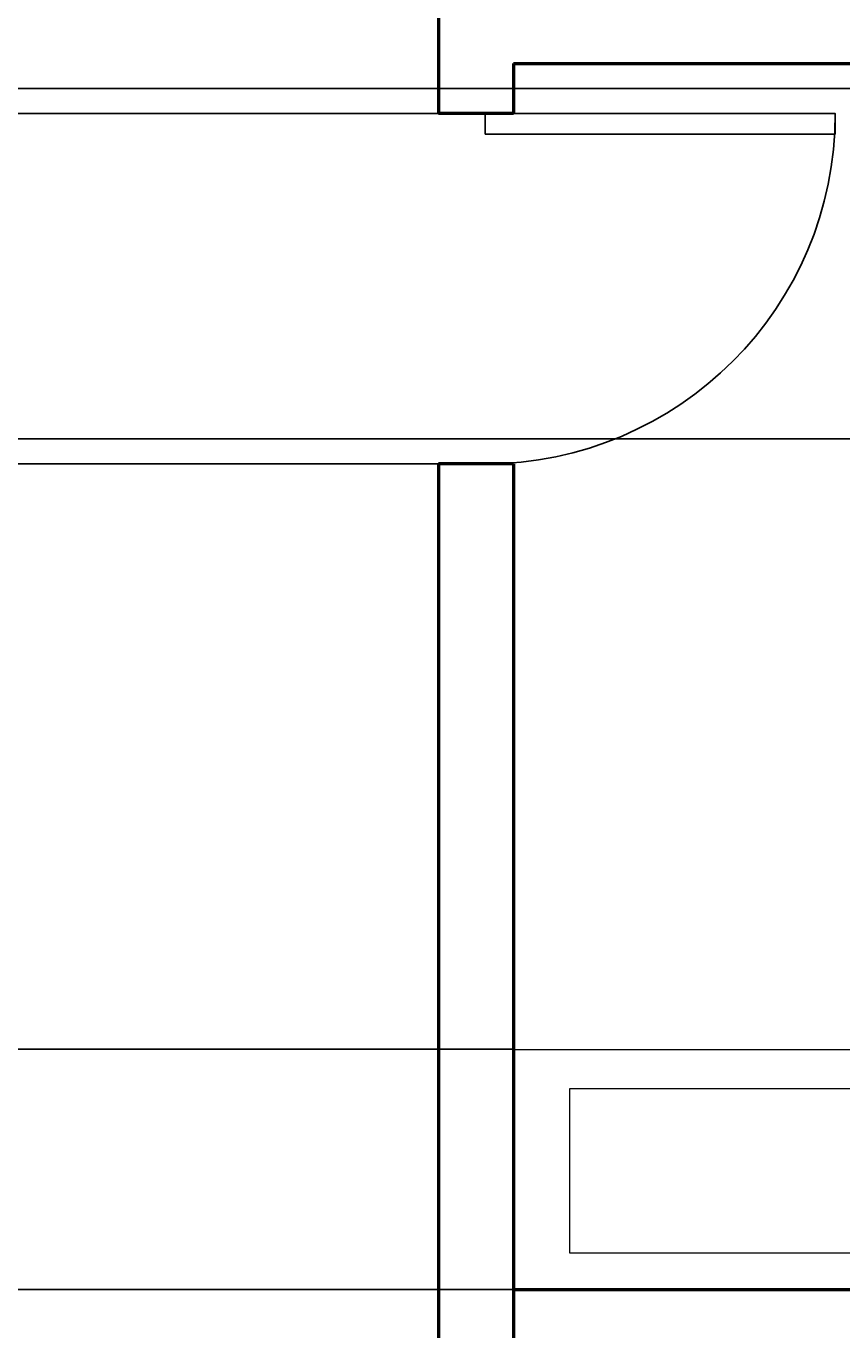
# Model space of a CAD drawing. Units: inches. Extents: x 5375 to 6084, y 16106 to 17259.
# Tile 27 of 32: x 5768 to 5866, y 16776 to 16932. Entities that reach past the tile are written whole.
import ezdxf

# ---------------------------------------------------------------- set-up
doc = ezdxf.new("R2010")
doc.units = ezdxf.units.IN
for name, color, linetype, lineweight in [('A-ANNO-DIMS', 2, 'Continuous', 18), ('A-FLOR-CASE', 3, 'Continuous', 18), ('A-FLOR-FIXT', 3, 'Continuous', 18), ('DOOR', 4, 'Continuous', 25), ('WALL', 6, 'Continuous', 50)]:
    doc.layers.add(name, color=color, linetype=linetype, lineweight=lineweight)
doc.styles.get("Standard").update_dxf_attribs({"font": 'arial.ttf'})
doc.dimstyles.get("Standard").update_dxf_attribs({"dimtxt": 0.18, "dimasz": 0.18, "dimexe": 0.18, "dimexo": 0.0625, "dimgap": 0.09, "dimtad": 0, "dimtih": 1, "dimtoh": 1, "dimdec": 4, "dimzin": 0, "dimdsep": 46, "dimtxsty": 'Standard', "dimcen": 0.09, "dimadec": 0, "dimazin": 0, "dimtfac": 1, "dimtdec": 4, "dimtofl": 0, "dimtmove": 0, "dimatfit": 3, "dimfxl": 1, "dimtolj": 1, "dimtzin": 0, "dimarcsym": 0})

# ---------------------------------------------------------------- blocks, each defined once
blk = doc.blocks.new('*U2')
for p, q in [((0, 0), (0, -100)), ((750, 0), (750, -100))]:
    blk.add_line(p, q)
blk.add_lwpolyline([(0, 0), (0, 750), (43.75, 750), (43.75, 0)], close=True)
blk.add_arc((0, 0), 750, 0, 90)
blk = doc.blocks.new('*D41')
at = {"layer": 'A-ANNO-DIMS', "color": 0, "lineweight": -2, "transparency": 16777216}
for p, q in [((5702.18, 16924.58), (6084.2, 16924.58)), ((6084.02, 16924.4), (6084.02, 16903.76)), ((6084.02, 16882.76), (6084.02, 16903.4)), ((5702.18, 16882.58), (6084.2, 16882.58))]:
    blk.add_line(p, q, dxfattribs=at)
at = {"layer": 'A-ANNO-DIMS', "color": 0, "transparency": 16777216}
for points in [[(6083.99, 16924.4), (6084.05, 16924.4), (6084.02, 16924.58)], [(6083.99, 16882.76), (6084.05, 16882.76), (6084.02, 16882.58)]]:
    blk.add_solid(points, dxfattribs=at)
at = {"layer": 'Defpoints', "color": 0, "transparency": 16777216}
for p in [(5702.12, 16924.58), (6084.02, 16924.58), (5702.12, 16882.58)]:
    blk.add_point(p, dxfattribs=at)
at = {"layer": 'A-ANNO-DIMS', "color": 0, "transparency": 16777216, "insert": (6084.02, 16903.58), "char_height": 0.18, "attachment_point": 5}
blk.add_mtext('\\A1;42', dxfattribs=at)
blk = doc.blocks.new('*D42')
at = {"layer": 'A-ANNO-DIMS', "color": 0, "lineweight": -2, "transparency": 16777216}
for p, q in [((5826.06, 16921.58), (5375.56, 16921.58)), ((5375.74, 16921.4), (5375.74, 16900.76)), ((5375.74, 16879.76), (5375.74, 16900.4)), ((5826.06, 16879.58), (5375.56, 16879.58))]:
    blk.add_line(p, q, dxfattribs=at)
at = {"layer": 'A-ANNO-DIMS', "color": 0, "transparency": 16777216}
for points in [[(5375.71, 16921.4), (5375.77, 16921.4), (5375.74, 16921.58)], [(5375.71, 16879.76), (5375.77, 16879.76), (5375.74, 16879.58)]]:
    blk.add_solid(points, dxfattribs=at)
at = {"layer": 'Defpoints', "color": 0, "transparency": 16777216}
for p in [(5826.12, 16921.58), (5375.74, 16879.58), (5826.12, 16879.58)]:
    blk.add_point(p, dxfattribs=at)
at = {"layer": 'A-ANNO-DIMS', "color": 0, "transparency": 16777216, "insert": (5375.74, 16900.58), "char_height": 0.18, "attachment_point": 5}
blk.add_mtext('\\A1;42', dxfattribs=at)
blk = doc.blocks.new('*D43')
at = {"layer": 'A-ANNO-DIMS', "color": 0, "lineweight": -2, "transparency": 16777216}
for p, q in [((5826.06, 16809.37), (5375.56, 16809.37)), ((5375.74, 16809.19), (5375.74, 16795.15)), ((5375.74, 16780.76), (5375.74, 16794.79)), ((5826.06, 16780.58), (5375.56, 16780.58))]:
    blk.add_line(p, q, dxfattribs=at)
at = {"layer": 'A-ANNO-DIMS', "color": 0, "transparency": 16777216}
for points in [[(5375.71, 16809.19), (5375.77, 16809.19), (5375.74, 16809.37)], [(5375.71, 16780.76), (5375.77, 16780.76), (5375.74, 16780.58)]]:
    blk.add_solid(points, dxfattribs=at)
at = {"layer": 'Defpoints', "color": 0, "transparency": 16777216}
for p in [(5375.74, 16809.37), (5826.12, 16809.37), (5826.12, 16780.58)]:
    blk.add_point(p, dxfattribs=at)
at = {"layer": 'A-ANNO-DIMS', "color": 0, "transparency": 16777216, "insert": (5375.74, 16794.97), "char_height": 0.18, "attachment_point": 5}
blk.add_mtext('\\A1;28.786', dxfattribs=at)

msp = doc.modelspace()

# ---------------------------------------------------------------- linework, layer by layer
at = {"layer": 'A-FLOR-CASE'}
msp.add_line((5826.1199, 16809.3651), (5914.0033, 16809.3651), dxfattribs=at)
at = {"layer": 'A-FLOR-FIXT'}
msp.add_lwpolyline([(5869.7591, 16784.9398), (5832.8693, 16784.9398), (5832.8693, 16804.67), (5869.7591, 16804.67)], close=True, dxfattribs=at)
at = {"layer": 'WALL'}
for p, q in [((5817.1199, 16936.5793), (5817.1199, 16921.5793)), ((5826.1199, 16927.5793), (5946.1199, 16927.5793)), ((5826.1199, 16927.5793), (5826.1199, 16921.5793)), ((5826.1199, 16921.5793), (5817.1199, 16921.5793)), ((5826.1199, 16879.5793), (5817.1199, 16879.5793)), ((5817.1199, 16879.5793), (5817.1199, 16699.5793)), ((5826.1199, 16879.5793), (5826.1199, 16699.5793)), ((5826.1199, 16780.5793), (5946.1199, 16780.5793))]:
    msp.add_line(p, q, dxfattribs=at)

# ---------------------------------------------------------------- block references
at = {"layer": 'DOOR', "xscale": 0.0559999999999998, "yscale": 0.0559999999999998, "zscale": 0.0559999999999998, "rotation": 270}
msp.add_blockref('*U2', (5822.7199, 16921.5793), dxfattribs=at)

# ---------------------------------------------------------------- dimensions: what is measured, and where the dimension line sits
at = {"layer": 'A-ANNO-DIMS'}
for base, p1, p2, override, picture, middle in [((6084.0199, 16924.5793), (5702.1199, 16882.5793), (5702.1199, 16924.5793), {"dimdec": 0, "dimlfac": 1, "dimrnd": 0, "dimzin": 0, "dimdsep": 46, "dimlunit": 2}, '*D41', (6084.0199, 16903.5793)), ((5375.7423, 16879.5793), (5826.1199, 16921.5793), (5826.1199, 16879.5793), {"dimdec": 0, "dimlfac": 1, "dimrnd": 0, "dimzin": 0, "dimdsep": 46, "dimlunit": 2}, '*D42', (5375.7423, 16900.5793)), ((5375.7423, 16809.3651), (5826.1199, 16780.5793), (5826.1199, 16809.3651), {"dimdec": 3, "dimlfac": 1, "dimrnd": 0, "dimzin": 0, "dimdsep": 46, "dimlunit": 2}, '*D43', (5375.7423, 16794.9722))]:
    dim = msp.add_linear_dim(base=base, p1=p1, p2=p2, angle=90, dimstyle='Standard', override=override, dxfattribs=at)
    dim.commit()
    dim.dimension.update_dxf_attribs({"geometry": picture, "text_midpoint": middle})

doc.saveas('drawing.dxf')
